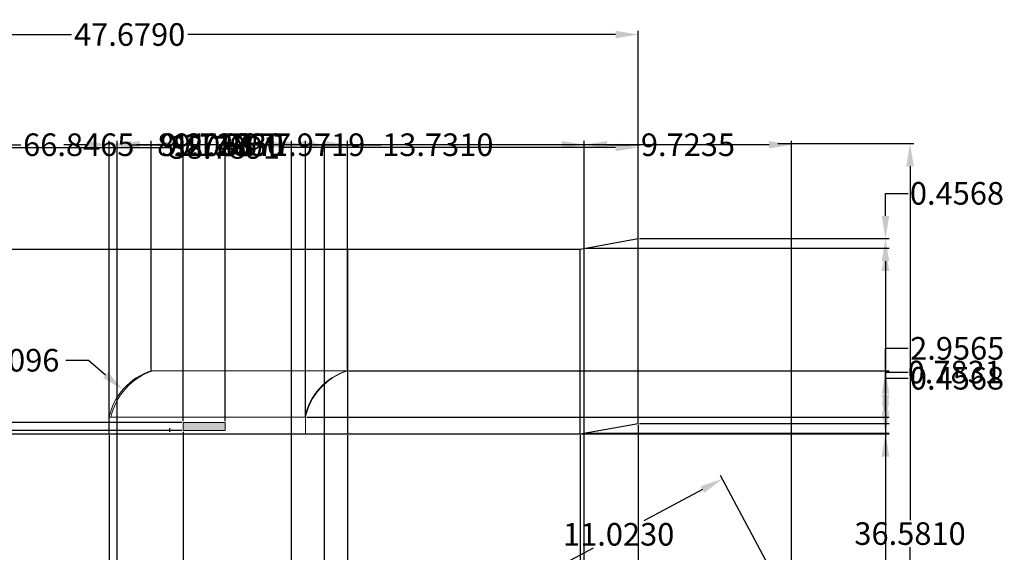
# Model space of a CAD drawing. Units: inches. Extents: x 32.3 to 119.3, y 11.9 to 64.
# Tile 3 of 3: x 73.2 to 119.3, y 39 to 64. Entities that reach past the tile are written whole.
import ezdxf

# ---------------------------------------------------------------- set-up
doc = ezdxf.new("R2010")
doc.units = ezdxf.units.IN
doc.header["$MEASUREMENT"] = 0
for name, color, linetype, lineweight in [('A-ANNO-DIMS', 2, 'Continuous', 18), ('A-EQPM', 4, 'Continuous', 18), ('A-EQPM-PATT', 8, 'Continuous', 13), ('A-FURN', 7, 'Continuous', 25)]:
    doc.layers.add(name, color=color, linetype=linetype, lineweight=lineweight)
doc.styles.get("Standard").update_dxf_attribs({"font": 'arial.ttf'})
doc.dimstyles.get("Standard").update_dxf_attribs({"dimtxt": 1.06, "dimasz": 1.06, "dimexe": 0.18, "dimexo": 0.0625, "dimgap": 0.09, "dimtad": 0, "dimtih": 1, "dimtoh": 1, "dimdec": 4, "dimzin": 0, "dimdsep": 46, "dimtxsty": 'Standard', "dimcen": 0.09, "dimadec": 0, "dimazin": 0, "dimtfac": 1, "dimtdec": 4, "dimtofl": 0, "dimtmove": 0, "dimatfit": 3, "dimfxl": 1, "dimtolj": 1, "dimtzin": 0, "dimarcsym": 0})

# ---------------------------------------------------------------- blocks, each defined once
blk = doc.blocks.new('*D1')
at = {"layer": 'A-ANNO-DIMS', "color": 0, "lineweight": -2, "transparency": 16777216}
for p, q in [((54.478, 52.49), (54.478, 63.441)), ((55.538, 63.261), (75.596, 63.261)), ((101.097, 63.261), (81.039, 63.261)), ((102.157, 52.49), (102.157, 63.441))]:
    blk.add_line(p, q, dxfattribs=at)
at = {"layer": 'A-ANNO-DIMS', "color": 0, "transparency": 16777216}
for points in [[(55.538, 63.438), (55.538, 63.085), (54.478, 63.261)], [(101.097, 63.438), (101.097, 63.085), (102.157, 63.261)]]:
    blk.add_solid(points, dxfattribs=at)
at = {"layer": 'Defpoints', "color": 0, "transparency": 16777216}
for p in [(102.157, 63.261), (54.478, 52.427), (102.157, 52.427)]:
    blk.add_point(p, dxfattribs=at)
at = {"layer": 'A-ANNO-DIMS', "color": 0, "transparency": 16777216, "insert": (78.318, 63.261), "char_height": 1.06, "attachment_point": 5}
blk.add_mtext('\\A1;47.6790', dxfattribs=at)
blk = doc.blocks.new('*D4')
at = {"layer": 'A-ANNO-DIMS', "color": 0, "lineweight": -2, "transparency": 16777216}
for p, q in [((63.368, 55.782), (63.368, 58.146)), ((64.428, 57.966), (80.163, 57.966)), ((101.097, 57.966), (85.362, 57.966)), ((102.157, 55.782), (102.157, 58.146))]:
    blk.add_line(p, q, dxfattribs=at)
at = {"layer": 'A-ANNO-DIMS', "color": 0, "transparency": 16777216}
for points in [[(64.428, 58.142), (64.428, 57.789), (63.368, 57.966)], [(101.097, 58.142), (101.097, 57.789), (102.157, 57.966)]]:
    blk.add_solid(points, dxfattribs=at)
at = {"layer": 'Defpoints', "color": 0, "transparency": 16777216}
for p in [(102.157, 57.966), (63.368, 55.72), (102.157, 55.72)]:
    blk.add_point(p, dxfattribs=at)
at = {"layer": 'A-ANNO-DIMS', "color": 0, "transparency": 16777216, "insert": (82.763, 57.966), "char_height": 1.06, "attachment_point": 5}
blk.add_mtext('\\A1;38.7891', dxfattribs=at)
blk = doc.blocks.new('*D10')
at = {"layer": 'A-ANNO-DIMS', "color": 0, "lineweight": -2, "transparency": 16777216}
for p, q in [((109.325, 36.391), (106.022, 42.576)), ((105.172, 41.918), (102.428, 40.453)), ((97.318, 37.724), (100.062, 39.19)), ((99.602, 31.198), (96.298, 37.384))]:
    blk.add_line(p, q, dxfattribs=at)
at = {"layer": 'A-ANNO-DIMS', "color": 0, "transparency": 16777216}
for points in [[(105.088, 42.074), (105.255, 41.762), (106.107, 42.418)], [(97.235, 37.88), (97.401, 37.569), (96.383, 37.225)]]:
    blk.add_solid(points, dxfattribs=at)
at = {"layer": 'Defpoints', "color": 0, "transparency": 16777216}
for p in [(106.107, 42.418), (109.354, 36.335), (99.631, 31.143)]:
    blk.add_point(p, dxfattribs=at)
at = {"layer": 'A-ANNO-DIMS', "color": 0, "transparency": 16777216, "insert": (101.245, 39.821), "char_height": 1.06, "attachment_point": 5}
blk.add_mtext('\\A1;11.0230', dxfattribs=at)
blk = doc.blocks.new('*D11')
at = {"layer": 'A-ANNO-DIMS', "color": 0, "lineweight": -2, "transparency": 16777216}
for p, q in [((108.706, 58.146), (115.085, 58.146)), ((114.905, 57.086), (114.905, 40.487)), ((114.905, 22.625), (114.905, 39.223)), ((108.706, 21.565), (115.085, 21.565))]:
    blk.add_line(p, q, dxfattribs=at)
at = {"layer": 'A-ANNO-DIMS', "color": 0, "transparency": 16777216}
for points in [[(114.729, 57.086), (115.082, 57.086), (114.905, 58.146)], [(114.729, 22.625), (115.082, 22.625), (114.905, 21.565)]]:
    blk.add_solid(points, dxfattribs=at)
at = {"layer": 'Defpoints', "color": 0, "transparency": 16777216}
for p in [(108.644, 58.146), (114.905, 58.146), (108.644, 21.565)]:
    blk.add_point(p, dxfattribs=at)
at = {"layer": 'A-ANNO-DIMS', "color": 0, "transparency": 16777216, "insert": (114.905, 39.855), "char_height": 1.06, "attachment_point": 5}
blk.add_mtext('\\A1;36.5810', dxfattribs=at)
blk = doc.blocks.new('*D12')
at = {"layer": 'A-ANNO-DIMS', "color": 0, "lineweight": -2, "transparency": 16777216}
for p, q in [((42.508, 51.967), (42.508, 58.272)), ((109.354, 36.398), (109.354, 58.272)), ((43.568, 58.092), (73.222, 58.092)), ((108.294, 58.092), (78.64, 58.092))]:
    blk.add_line(p, q, dxfattribs=at)
at = {"layer": 'A-ANNO-DIMS', "color": 0, "transparency": 16777216}
for points in [[(43.568, 58.269), (43.568, 57.916), (42.508, 58.092)], [(108.294, 58.269), (108.294, 57.916), (109.354, 58.092)]]:
    blk.add_solid(points, dxfattribs=at)
at = {"layer": 'Defpoints', "color": 0, "transparency": 16777216}
for p in [(109.354, 58.092), (42.508, 51.905), (109.354, 36.335)]:
    blk.add_point(p, dxfattribs=at)
at = {"layer": 'A-ANNO-DIMS', "color": 0, "transparency": 16777216, "insert": (75.931, 58.092), "char_height": 1.06, "attachment_point": 5}
blk.add_mtext('\\A1;66.8465', dxfattribs=at)
blk = doc.blocks.new('*D23')
at = {"layer": 'A-ANNO-DIMS', "color": 0, "lineweight": -2, "transparency": 16777216}
for p, q in [((102.22, 53.692), (113.934, 53.692)), ((113.754, 52.632), (113.754, 35.971)), ((113.754, 18.046), (113.754, 34.708)), ((99.726, 16.986), (113.934, 16.986))]:
    blk.add_line(p, q, dxfattribs=at)
at = {"layer": 'A-ANNO-DIMS', "color": 0, "transparency": 16777216}
for points in [[(113.578, 52.632), (113.931, 52.632), (113.754, 53.692)], [(113.578, 18.046), (113.931, 18.046), (113.754, 16.986)]]:
    blk.add_solid(points, dxfattribs=at)
at = {"layer": 'Defpoints', "color": 0, "transparency": 16777216}
for p in [(102.157, 53.692), (113.754, 53.692), (99.664, 16.986)]:
    blk.add_point(p, dxfattribs=at)
at = {"layer": 'A-ANNO-DIMS', "color": 0, "transparency": 16777216, "insert": (113.754, 35.339), "char_height": 1.06, "attachment_point": 5}
blk.add_mtext('\\A1;36.7068', dxfattribs=at)
blk = doc.blocks.new('*D26')
at = {"layer": 'A-ANNO-DIMS', "color": 0, "lineweight": -2, "transparency": 16777216}
for p, q in [((77.355, 45.373), (77.355, 58.272)), ((88.528, 47.546), (88.528, 58.272)), ((78.415, 58.092), (80.292, 58.092)), ((87.468, 58.092), (85.592, 58.092))]:
    blk.add_line(p, q, dxfattribs=at)
at = {"layer": 'A-ANNO-DIMS', "color": 0, "transparency": 16777216}
for points in [[(78.415, 58.269), (78.415, 57.916), (77.355, 58.092)], [(87.468, 58.269), (87.468, 57.916), (88.528, 58.092)]]:
    blk.add_solid(points, dxfattribs=at)
at = {"layer": 'Defpoints', "color": 0, "transparency": 16777216}
for p in [(88.528, 58.092), (88.528, 47.484), (77.355, 45.31)]:
    blk.add_point(p, dxfattribs=at)
at = {"layer": 'A-ANNO-DIMS', "color": 0, "transparency": 16777216, "insert": (82.942, 58.092), "char_height": 1.06, "attachment_point": 5}
blk.add_mtext('\\A1;11.1730', dxfattribs=at)
blk = doc.blocks.new('*D27')
at = {"layer": 'A-ANNO-DIMS', "color": 0, "lineweight": -2, "transparency": 16777216}
for p, q in [((88.528, 44.465), (88.528, 12.388)), ((99.437, 44.465), (99.437, 12.388)), ((89.588, 12.568), (91.33, 12.568)), ((98.377, 12.568), (96.636, 12.568))]:
    blk.add_line(p, q, dxfattribs=at)
at = {"layer": 'A-ANNO-DIMS', "color": 0, "transparency": 16777216}
for points in [[(89.588, 12.745), (89.588, 12.391), (88.528, 12.568)], [(98.377, 12.745), (98.377, 12.391), (99.437, 12.568)]]:
    blk.add_solid(points, dxfattribs=at)
at = {"layer": 'Defpoints', "color": 0, "transparency": 16777216}
for p in [(88.528, 44.527), (99.437, 44.527), (99.437, 12.568)]:
    blk.add_point(p, dxfattribs=at)
at = {"layer": 'A-ANNO-DIMS', "color": 0, "transparency": 16777216, "insert": (93.983, 12.568), "char_height": 1.06, "attachment_point": 5}
blk.add_mtext('\\A1;10.9088', dxfattribs=at)
blk = doc.blocks.new('*D28')
at = {"layer": 'A-ANNO-DIMS', "color": 0, "lineweight": -2, "transparency": 16777216}
for p, q in [((102.157, 44.957), (102.157, 12.388)), ((99.437, 44.465), (99.437, 12.388)), ((100.497, 12.568), (101.097, 12.568)), ((102.157, 12.568), (103.217, 12.568))]:
    blk.add_line(p, q, dxfattribs=at)
at = {"layer": 'A-ANNO-DIMS', "color": 0, "transparency": 16777216}
for points in [[(100.497, 12.745), (100.497, 12.391), (99.437, 12.568)], [(101.097, 12.745), (101.097, 12.391), (102.157, 12.568)]]:
    blk.add_solid(points, dxfattribs=at)
at = {"layer": 'Defpoints', "color": 0, "transparency": 16777216}
for p in [(102.157, 45.02), (99.437, 44.527), (102.157, 12.568)]:
    blk.add_point(p, dxfattribs=at)
at = {"layer": 'A-ANNO-DIMS', "color": 0, "transparency": 16777216, "insert": (105.414, 12.568), "char_height": 1.06, "attachment_point": 5}
blk.add_mtext('\\A1;2.7201', dxfattribs=at)
blk = doc.blocks.new('*D29')
at = {"layer": 'A-ANNO-DIMS', "color": 0, "lineweight": -2, "transparency": 16777216}
for p, q in [((113.754, 54.752), (113.754, 55.812)), ((113.754, 55.812), (114.814, 55.812)), ((102.22, 53.692), (113.934, 53.692)), ((99.696, 53.236), (113.934, 53.236)), ((113.754, 52.176), (113.754, 51.116))]:
    blk.add_line(p, q, dxfattribs=at)
at = {"layer": 'A-ANNO-DIMS', "color": 0, "transparency": 16777216}
for points in [[(113.578, 54.752), (113.931, 54.752), (113.754, 53.692)], [(113.578, 52.176), (113.931, 52.176), (113.754, 53.236)]]:
    blk.add_solid(points, dxfattribs=at)
at = {"layer": 'Defpoints', "color": 0, "transparency": 16777216}
for p in [(102.157, 53.692), (113.754, 53.692), (99.634, 53.236)]:
    blk.add_point(p, dxfattribs=at)
at = {"layer": 'A-ANNO-DIMS', "color": 0, "transparency": 16777216, "insert": (117.106, 55.812), "char_height": 1.06, "attachment_point": 5}
blk.add_mtext('\\A1;0.4568', dxfattribs=at)
blk = doc.blocks.new('*D30')
at = {"layer": 'A-ANNO-DIMS', "color": 0, "lineweight": -2, "transparency": 16777216}
for p, q in [((113.754, 46.08), (113.754, 47.14)), ((113.754, 47.14), (114.814, 47.14)), ((102.22, 45.02), (113.934, 45.02)), ((99.696, 44.563), (113.934, 44.563)), ((113.754, 43.503), (113.754, 42.443))]:
    blk.add_line(p, q, dxfattribs=at)
at = {"layer": 'A-ANNO-DIMS', "color": 0, "transparency": 16777216}
for points in [[(113.578, 46.08), (113.931, 46.08), (113.754, 45.02)], [(113.578, 43.503), (113.931, 43.503), (113.754, 44.563)]]:
    blk.add_solid(points, dxfattribs=at)
at = {"layer": 'Defpoints', "color": 0, "transparency": 16777216}
for p in [(102.157, 45.02), (113.754, 45.02), (99.634, 44.563)]:
    blk.add_point(p, dxfattribs=at)
at = {"layer": 'A-ANNO-DIMS', "color": 0, "transparency": 16777216, "insert": (117.106, 47.14), "char_height": 1.06, "attachment_point": 5}
blk.add_mtext('\\A1;0.4568', dxfattribs=at)
blk = doc.blocks.new('*D34')
at = {"layer": 'A-ANNO-DIMS', "color": 0, "lineweight": -2, "transparency": 16777216}
for p, q in [((113.754, 47.484), (113.754, 48.544)), ((113.754, 48.544), (114.814, 48.544)), ((88.591, 47.484), (113.934, 47.484)), ((113.754, 45.587), (113.754, 46.424)), ((88.591, 44.527), (113.934, 44.527))]:
    blk.add_line(p, q, dxfattribs=at)
at = {"layer": 'A-ANNO-DIMS', "color": 0, "transparency": 16777216}
for points in [[(113.578, 46.424), (113.931, 46.424), (113.754, 47.484)], [(113.578, 45.587), (113.931, 45.587), (113.754, 44.527)]]:
    blk.add_solid(points, dxfattribs=at)
at = {"layer": 'Defpoints', "color": 0, "transparency": 16777216}
for p in [(88.528, 47.484), (113.754, 47.484), (88.528, 44.527)]:
    blk.add_point(p, dxfattribs=at)
at = {"layer": 'A-ANNO-DIMS', "color": 0, "transparency": 16777216, "insert": (117.118, 48.544), "char_height": 1.06, "attachment_point": 5}
blk.add_mtext('\\A1;2.9565', dxfattribs=at)
blk = doc.blocks.new('*D35')
at = {"layer": 'A-ANNO-DIMS', "color": 0, "lineweight": -2, "transparency": 16777216}
for p, q in [((113.754, 46.37), (113.754, 47.43)), ((113.754, 47.43), (114.814, 47.43)), ((86.623, 45.31), (113.934, 45.31)), ((86.623, 44.527), (113.934, 44.527)), ((113.754, 43.467), (113.754, 42.407))]:
    blk.add_line(p, q, dxfattribs=at)
at = {"layer": 'A-ANNO-DIMS', "color": 0, "transparency": 16777216}
for points in [[(113.578, 46.37), (113.931, 46.37), (113.754, 45.31)], [(113.578, 43.467), (113.931, 43.467), (113.754, 44.527)]]:
    blk.add_solid(points, dxfattribs=at)
at = {"layer": 'Defpoints', "color": 0, "transparency": 16777216}
for p in [(86.561, 45.31), (113.754, 45.31), (86.561, 44.527)]:
    blk.add_point(p, dxfattribs=at)
at = {"layer": 'A-ANNO-DIMS', "color": 0, "transparency": 16777216, "insert": (117.002, 47.43), "char_height": 1.06, "attachment_point": 5}
blk.add_mtext('\\A1;0.7831', dxfattribs=at)
blk = doc.blocks.new('*D36')
at = {"layer": 'A-ANNO-DIMS', "color": 0, "lineweight": -2, "transparency": 16777216}
for p, q in [((77.355, 45.373), (77.355, 58.272)), ((86.561, 45.373), (86.561, 58.272)), ((78.415, 58.092), (79.668, 58.092)), ((85.501, 58.092), (84.248, 58.092))]:
    blk.add_line(p, q, dxfattribs=at)
at = {"layer": 'A-ANNO-DIMS', "color": 0, "transparency": 16777216}
for points in [[(78.415, 58.269), (78.415, 57.916), (77.355, 58.092)], [(85.501, 58.269), (85.501, 57.916), (86.561, 58.092)]]:
    blk.add_solid(points, dxfattribs=at)
at = {"layer": 'Defpoints', "color": 0, "transparency": 16777216}
for p in [(86.561, 58.092), (77.355, 45.31), (86.561, 45.31)]:
    blk.add_point(p, dxfattribs=at)
at = {"layer": 'A-ANNO-DIMS', "color": 0, "transparency": 16777216, "insert": (81.958, 58.092), "char_height": 1.06, "attachment_point": 5}
blk.add_mtext('\\A1;9.2053', dxfattribs=at)
blk = doc.blocks.new('*D37')
at = {"layer": 'A-ANNO-DIMS', "color": 0, "lineweight": -2, "transparency": 16777216}
for p, q in [((77.355, 44.59), (77.355, 58.272)), ((79.323, 47.546), (79.323, 58.272)), ((76.295, 58.092), (75.235, 58.092)), ((80.383, 58.092), (81.443, 58.092))]:
    blk.add_line(p, q, dxfattribs=at)
at = {"layer": 'A-ANNO-DIMS', "color": 0, "transparency": 16777216}
for points in [[(76.295, 58.269), (76.295, 57.916), (77.355, 58.092)], [(80.383, 58.269), (80.383, 57.916), (79.323, 58.092)]]:
    blk.add_solid(points, dxfattribs=at)
at = {"layer": 'Defpoints', "color": 0, "transparency": 16777216}
for p in [(79.323, 58.092), (79.323, 47.484), (77.355, 44.527)]:
    blk.add_point(p, dxfattribs=at)
at = {"layer": 'A-ANNO-DIMS', "color": 0, "transparency": 16777216, "insert": (83.683, 58.092), "char_height": 1.06, "attachment_point": 5}
blk.add_mtext('\\A1;1.9677', dxfattribs=at)
blk = doc.blocks.new('*D38')
at = {"layer": 'A-ANNO-DIMS', "color": 0, "lineweight": -2, "transparency": 16777216}
for p, q in [((80.821, 45.121), (80.821, 58.272)), ((82.793, 45.121), (82.793, 58.272)), ((79.761, 58.092), (78.701, 58.092)), ((83.853, 58.092), (84.913, 58.092))]:
    blk.add_line(p, q, dxfattribs=at)
at = {"layer": 'A-ANNO-DIMS', "color": 0, "transparency": 16777216}
for points in [[(79.761, 58.269), (79.761, 57.916), (80.821, 58.092)], [(83.853, 58.269), (83.853, 57.916), (82.793, 58.092)]]:
    blk.add_solid(points, dxfattribs=at)
at = {"layer": 'Defpoints', "color": 0, "transparency": 16777216}
for p in [(82.793, 58.092), (80.821, 45.059), (82.793, 45.059)]:
    blk.add_point(p, dxfattribs=at)
at = {"layer": 'A-ANNO-DIMS', "color": 0, "transparency": 16777216, "insert": (87.154, 58.092), "char_height": 1.06, "attachment_point": 5}
blk.add_mtext('\\A1;1.9719', dxfattribs=at)
blk = doc.blocks.new('*D39')
at = {"layer": 'A-ANNO-DIMS', "color": 0, "lineweight": -2, "transparency": 16777216}
for p, q in [((77.355, 44.465), (77.355, 12.388)), ((80.821, 44.632), (80.821, 12.388)), ((78.415, 12.568), (79.761, 12.568)), ((80.821, 12.568), (81.881, 12.568))]:
    blk.add_line(p, q, dxfattribs=at)
at = {"layer": 'A-ANNO-DIMS', "color": 0, "transparency": 16777216}
for points in [[(78.415, 12.745), (78.415, 12.391), (77.355, 12.568)], [(79.761, 12.745), (79.761, 12.391), (80.821, 12.568)]]:
    blk.add_solid(points, dxfattribs=at)
at = {"layer": 'Defpoints', "color": 0, "transparency": 16777216}
for p in [(77.355, 44.527), (80.821, 44.694), (80.821, 12.568)]:
    blk.add_point(p, dxfattribs=at)
at = {"layer": 'A-ANNO-DIMS', "color": 0, "transparency": 16777216, "insert": (84.17, 12.568), "char_height": 1.06, "attachment_point": 5}
blk.add_mtext('\\A1;3.4656', dxfattribs=at)
blk = doc.blocks.new('*D40')
at = {"layer": 'A-ANNO-DIMS', "color": 0, "lineweight": -2, "transparency": 16777216}
for p, q in [((38.108, 46.119), (38.108, 47.179)), ((38.108, 47.179), (39.168, 47.179)), ((80.758, 45.059), (37.928, 45.059)), ((80.758, 44.694), (37.928, 44.694)), ((38.108, 43.634), (38.108, 42.574))]:
    blk.add_line(p, q, dxfattribs=at)
at = {"layer": 'A-ANNO-DIMS', "color": 0, "transparency": 16777216}
for points in [[(37.931, 46.119), (38.285, 46.119), (38.108, 45.059)], [(37.931, 43.634), (38.285, 43.634), (38.108, 44.694)]]:
    blk.add_solid(points, dxfattribs=at)
at = {"layer": 'Defpoints', "color": 0, "transparency": 16777216}
for p in [(38.108, 45.059), (80.821, 45.059), (80.821, 44.694)]:
    blk.add_point(p, dxfattribs=at)
at = {"layer": 'A-ANNO-DIMS', "color": 0, "transparency": 16777216, "insert": (41.458, 47.179), "char_height": 1.06, "attachment_point": 5}
blk.add_mtext('\\A1;0.3643', dxfattribs=at)
blk = doc.blocks.new('*D45')
at = {"layer": 'A-ANNO-DIMS', "color": 0, "lineweight": -2, "transparency": 16777216}
for p, q in [((77.725, 31.206), (77.725, 58.272)), ((85.9, 31.206), (85.9, 58.272)), ((78.785, 58.092), (79.521, 58.092)), ((84.84, 58.092), (84.105, 58.092))]:
    blk.add_line(p, q, dxfattribs=at)
at = {"layer": 'A-ANNO-DIMS', "color": 0, "transparency": 16777216}
for points in [[(78.785, 58.269), (78.785, 57.916), (77.725, 58.092)], [(84.84, 58.269), (84.84, 57.916), (85.9, 58.092)]]:
    blk.add_solid(points, dxfattribs=at)
at = {"layer": 'Defpoints', "color": 0, "transparency": 16777216}
for p in [(85.9, 58.092), (77.725, 31.143), (85.9, 31.143)]:
    blk.add_point(p, dxfattribs=at)
at = {"layer": 'A-ANNO-DIMS', "color": 0, "transparency": 16777216, "insert": (81.813, 58.092), "char_height": 1.06, "attachment_point": 5}
blk.add_mtext('\\A1;8.1748', dxfattribs=at)
blk = doc.blocks.new('*D46')
at = {"layer": 'A-ANNO-DIMS', "color": 0, "lineweight": -2, "transparency": 16777216}
for p, q in [((77.725, 31.206), (77.725, 58.272)), ((87.449, 36.398), (87.449, 58.272)), ((78.785, 58.092), (80.293, 58.092)), ((86.389, 58.092), (84.881, 58.092))]:
    blk.add_line(p, q, dxfattribs=at)
at = {"layer": 'A-ANNO-DIMS', "color": 0, "transparency": 16777216}
for points in [[(78.785, 58.269), (78.785, 57.916), (77.725, 58.092)], [(86.389, 58.269), (86.389, 57.916), (87.449, 58.092)]]:
    blk.add_solid(points, dxfattribs=at)
at = {"layer": 'Defpoints', "color": 0, "transparency": 16777216}
for p in [(87.449, 58.092), (87.449, 36.335), (77.725, 31.143)]:
    blk.add_point(p, dxfattribs=at)
at = {"layer": 'A-ANNO-DIMS', "color": 0, "transparency": 16777216, "insert": (82.587, 58.092), "char_height": 1.06, "attachment_point": 5}
blk.add_mtext('\\A1;9.7235', dxfattribs=at)
blk = doc.blocks.new('*D47')
at = {"layer": 'A-ANNO-DIMS', "color": 0, "lineweight": -2, "transparency": 16777216}
for p, q in [((85.9, 31.206), (85.9, 58.272)), ((99.631, 31.206), (99.631, 58.272)), ((86.96, 58.092), (90.115, 58.092)), ((98.571, 58.092), (95.416, 58.092))]:
    blk.add_line(p, q, dxfattribs=at)
at = {"layer": 'A-ANNO-DIMS', "color": 0, "transparency": 16777216}
for points in [[(86.96, 58.269), (86.96, 57.916), (85.9, 58.092)], [(98.571, 58.269), (98.571, 57.916), (99.631, 58.092)]]:
    blk.add_solid(points, dxfattribs=at)
at = {"layer": 'Defpoints', "color": 0, "transparency": 16777216}
for p in [(99.631, 58.092), (85.9, 31.143), (99.631, 31.143)]:
    blk.add_point(p, dxfattribs=at)
at = {"layer": 'A-ANNO-DIMS', "color": 0, "transparency": 16777216, "insert": (92.765, 58.092), "char_height": 1.06, "attachment_point": 5}
blk.add_mtext('\\A1;13.7310', dxfattribs=at)
blk = doc.blocks.new('*D48')
at = {"layer": 'A-ANNO-DIMS', "color": 0, "lineweight": -2, "transparency": 16777216}
for p, q in [((99.631, 31.206), (99.631, 58.272)), ((109.354, 36.398), (109.354, 58.272)), ((100.691, 58.092), (102.198, 58.092)), ((108.294, 58.092), (106.787, 58.092))]:
    blk.add_line(p, q, dxfattribs=at)
at = {"layer": 'A-ANNO-DIMS', "color": 0, "transparency": 16777216}
for points in [[(100.691, 58.269), (100.691, 57.916), (99.631, 58.092)], [(108.294, 58.269), (108.294, 57.916), (109.354, 58.092)]]:
    blk.add_solid(points, dxfattribs=at)
at = {"layer": 'Defpoints', "color": 0, "transparency": 16777216}
for p in [(109.354, 58.092), (109.354, 36.335), (99.631, 31.143)]:
    blk.add_point(p, dxfattribs=at)
at = {"layer": 'A-ANNO-DIMS', "color": 0, "transparency": 16777216, "insert": (104.493, 58.092), "char_height": 1.06, "attachment_point": 5}
blk.add_mtext('\\A1;9.7235', dxfattribs=at)
blk = doc.blocks.new('*D61')
at = {"layer": 'A-ANNO-DIMS', "color": 0, "lineweight": -2, "transparency": 16777216}
for p, q in [((75.325, 47.985), (76.385, 47.985)), ((76.385, 47.985), (77.19, 47.295)), ((80.202, 44.62), (80.202, 44.8)), ((80.112, 44.71), (80.292, 44.71))]:
    blk.add_line(p, q, dxfattribs=at)
at = {"layer": 'A-ANNO-DIMS', "color": 0, "transparency": 16777216}
blk.add_solid([(77.305, 47.429), (77.075, 47.161), (77.994, 46.605)], dxfattribs=at)
at = {"layer": 'Defpoints', "color": 0, "transparency": 16777216}
for p in [(77.994, 46.605), (80.202, 44.71)]:
    blk.add_point(p, dxfattribs=at)
at = {"layer": 'A-ANNO-DIMS', "color": 0, "transparency": 16777216, "insert": (71.38, 47.985), "char_height": 1.06, "attachment_point": 5}
blk.add_mtext('\\A1;2X R2.9096', dxfattribs=at)

msp = doc.modelspace()

# ---------------------------------------------------------------- hatches: boundary and pattern name
at = {"layer": 'A-EQPM-PATT'}
h = msp.add_hatch(color=256, dxfattribs=at)
h.dxf.hatch_style = 1
h.paths.add_polyline_path([(82.7928, 45.05867), (80.82094, 45.05867), (80.82094, 44.6944), (82.7928, 44.6944)])

# ---------------------------------------------------------------- linework, layer by layer
at = {"layer": 'A-EQPM'}
for p, q in [((79.32312, 47.48385), (79.32312, 53.20007)), ((79.32312, 47.48385), (88.52838, 47.48385)), ((77.35538, 44.52731), (77.35538, 45.31043)), ((77.35538, 45.31043), (86.56064, 45.31043)), ((86.56064, 45.31043), (86.56064, 44.52731))]:
    msp.add_line(p, q, dxfattribs=at)
msp.add_lwpolyline([(80.82094, 45.05867), (82.7928, 45.05867), (82.7928, 44.6944), (80.82094, 44.6944)], close=True, dxfattribs=at)
for centre in [(80.20238, 44.71033), (80.28744, 44.71033), (89.37488, 44.71033), (89.40764, 44.71033)]:
    msp.add_arc(centre, 2.90956, 107.589622, 168.097254, dxfattribs=at)
at = {"layer": 'A-FURN'}
for p, q in [((99.43717, 53.20007), (102.15728, 53.69249)), ((102.15728, 45.01973), (102.15728, 53.69249)), ((59.20908, 53.20007), (99.43717, 53.20007)), ((88.52838, 53.20007), (88.52838, 44.52731)), ((99.43717, 44.52731), (99.43717, 53.20007)), ((99.63377, 44.5629), (99.63377, 53.23566)), ((99.43717, 44.52731), (102.15728, 45.01973)), ((59.20908, 44.52731), (99.43717, 44.52731))]:
    msp.add_line(p, q, dxfattribs=at)

# ---------------------------------------------------------------- dimensions: what is measured, and where the dimension line sits
at = {"layer": 'A-ANNO-DIMS'}
for base, p1, p2, override, picture, middle in [((102.15728, 63.26132), (54.4783, 52.42729), (102.15728, 52.42729), {"dimclrd": 0, "dimclre": 0, "dimclrt": 0}, '*D1', (78.31779, 63.26132)), ((109.35445, 58.09249), (42.50795, 51.90451), (109.35445, 36.33549), {"dimdec": 4, "dimlfac": 1, "dimrnd": 0, "dimzin": 0, "dimdsep": 46, "dimlunit": 2}, '*D12', (75.9312, 58.09249)), ((102.15728, 57.96555), (63.36818, 55.71994), (102.15728, 55.71994), {"dimclrd": 0, "dimclre": 0, "dimclrt": 0}, '*D4', (82.76273, 57.96555)), ((79.32312, 58.09249), (77.35538, 44.52731), (79.32312, 47.48385), {"dimdec": 4, "dimlfac": 1, "dimrnd": 0, "dimzin": 0, "dimdsep": 46, "dimlunit": 2}, '*D37', (83.68349, 58.09249)), ((88.52838, 58.09249), (77.35538, 45.31043), (88.52838, 47.48385), {"dimdec": 4, "dimlfac": 1, "dimrnd": 0, "dimzin": 0, "dimdsep": 46, "dimlunit": 2}, '*D26', (82.94188, 58.09249)), ((86.56064, 58.09249), (77.35538, 45.31043), (86.56064, 45.31043), {"dimdec": 4, "dimlfac": 1, "dimrnd": 0, "dimzin": 0, "dimdsep": 46, "dimlunit": 2}, '*D36', (81.95801, 58.09249)), ((85.89997, 58.09249), (77.72517, 31.14308), (85.89997, 31.14308), {"dimdec": 4, "dimlfac": 1, "dimrnd": 0, "dimzin": 0, "dimdsep": 46, "dimlunit": 2}, '*D45', (81.81257, 58.09249)), ((87.44863, 58.09249), (77.72517, 31.14308), (87.44863, 36.33549), {"dimdec": 4, "dimlfac": 1, "dimrnd": 0, "dimzin": 0, "dimdsep": 46, "dimlunit": 2}, '*D46', (82.5869, 58.09249)), ((82.7928, 58.09249), (80.82094, 45.05867), (82.7928, 45.05867), {"dimdec": 4, "dimlfac": 1, "dimrnd": 0, "dimzin": 0, "dimdsep": 46, "dimlunit": 2}, '*D38', (87.15425, 58.09249)), ((99.63098, 58.09249), (85.89997, 31.14308), (99.63098, 31.14308), {"dimdec": 4, "dimlfac": 1, "dimrnd": 0, "dimzin": 0, "dimdsep": 46, "dimlunit": 2}, '*D47', (92.76548, 58.09249)), ((109.35445, 58.09249), (99.63098, 31.14308), (109.35445, 36.33549), {"dimdec": 4, "dimlfac": 1, "dimrnd": 0, "dimzin": 0, "dimdsep": 46, "dimlunit": 2}, '*D48', (104.49272, 58.09249)), ((102.15728, 12.5681), (99.43717, 44.52731), (102.15728, 45.01973), {"dimdec": 4, "dimlfac": 1, "dimrnd": 0, "dimzin": 0, "dimdsep": 46, "dimlunit": 2}, '*D28', (105.41427, 12.5681)), ((80.82094, 12.5681), (77.35538, 44.52731), (80.82094, 44.6944), {"dimdec": 4, "dimlfac": 1, "dimrnd": 0, "dimzin": 0, "dimdsep": 46, "dimlunit": 2}, '*D39', (84.17048, 12.5681)), ((99.43717, 12.5681), (88.52838, 44.52731), (99.43717, 44.52731), {"dimdec": 4, "dimlfac": 1, "dimrnd": 0, "dimzin": 0, "dimdsep": 46, "dimlunit": 2}, '*D27', (93.98277, 12.5681))]:
    dim = msp.add_linear_dim(base=base, p1=p1, p2=p2, dimstyle='Standard', override=override, dxfattribs=at)
    dim.commit()
    dim.dimension.update_dxf_attribs({"geometry": picture, "text_midpoint": middle})
for base, p1, p2, override, picture, middle in [((114.90536, 58.14555), (108.6437, 21.56458), (108.6437, 58.14555), {"dimclrd": 0, "dimclre": 0, "dimclrt": 0}, '*D11', (114.90536, 39.85507)), ((113.75445, 53.69249), (99.63377, 53.23566), (102.15728, 53.69249), {"dimdec": 4, "dimlfac": 1, "dimrnd": 0, "dimzin": 0, "dimdsep": 46, "dimlunit": 2}, '*D29', (117.10579, 55.81249)), ((113.75445, 53.69249), (99.66386, 16.98566), (102.15728, 53.69249), {"dimdec": 4, "dimlfac": 1, "dimrnd": 0, "dimzin": 0, "dimdsep": 46, "dimlunit": 2}, '*D23', (113.75445, 35.33907)), ((113.75445, 47.48385), (88.52838, 44.52731), (88.52838, 47.48385), {"dimdec": 4, "dimlfac": 1, "dimrnd": 0, "dimzin": 0, "dimdsep": 46, "dimlunit": 2}, '*D34', (117.11772, 48.54385)), ((113.75445, 45.31043), (86.56064, 44.52731), (86.56064, 45.31043), {"dimdec": 4, "dimlfac": 1, "dimrnd": 0, "dimzin": 0, "dimdsep": 46, "dimlunit": 2}, '*D35', (117.00239, 47.43043)), ((38.10795, 45.05867), (80.82094, 44.6944), (80.82094, 45.05867), {"dimdec": 4, "dimlfac": 1, "dimrnd": 0, "dimzin": 0, "dimdsep": 46, "dimlunit": 2}, '*D40', (41.45821, 47.17867)), ((113.75445, 45.01973), (99.63377, 44.5629), (102.15728, 45.01973), {"dimdec": 4, "dimlfac": 1, "dimrnd": 0, "dimzin": 0, "dimdsep": 46, "dimlunit": 2}, '*D30', (117.10579, 47.13973))]:
    dim = msp.add_linear_dim(base=base, p1=p1, p2=p2, angle=90, dimstyle='Standard', override=override, dxfattribs=at)
    dim.commit()
    dim.dimension.update_dxf_attribs({"geometry": picture, "text_midpoint": middle})
dim = msp.add_radius_dim(center=(80.20238, 44.71033), mpoint=(77.99423, 46.60495), text='2X <>', dimstyle='Standard', override={"dimdec": 4, "dimlfac": 1, "dimrnd": 0, "dimzin": 0, "dimdsep": 46, "dimlunit": 2}, dxfattribs=at)
dim.commit()
dim.dimension.update_dxf_attribs({"geometry": '*D61', "text_midpoint": (71.38032, 47.98544)})
dim = msp.add_aligned_dim(p1=(99.63098, 31.14308), p2=(109.35445, 36.33549), distance=6.8949, dimstyle='Standard', override={"dimclrd": 0, "dimclre": 0, "dimclrt": 0}, dxfattribs=at)
dim.commit()
dim.dimension.update_dxf_attribs({"geometry": '*D10', "text_midpoint": (101.24486, 39.82132)})

doc.saveas('drawing.dxf')
